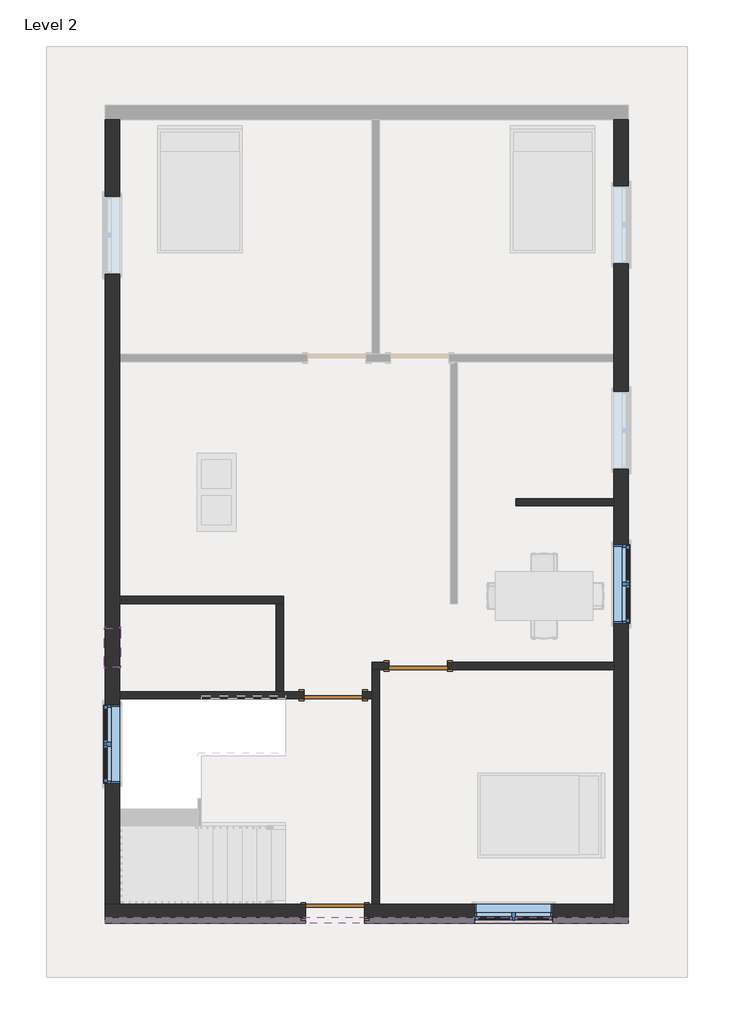
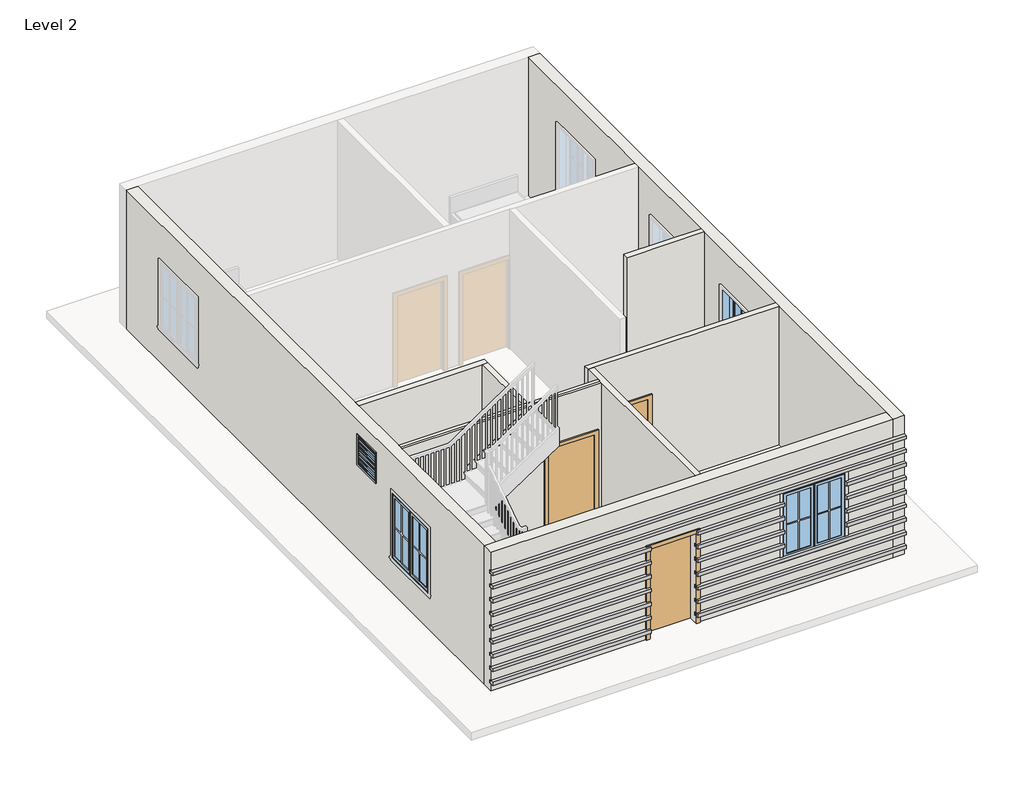
# One storey, part 1 of 3: 9 proxies, 9 walls, 4 windows, 3 doors.
"""IFC4 building model written with IfcOpenShell, lengths in millimetres."""

from ifc_helpers import new_model, si_unit, frame, origin, place, context, project, spatial, polyline, outline, extrude, faceted_brep, transform, mapped, element, save
from components import single_flush_door_3_17d80c48, single_flush_door_3_5e62189b, single_flush_door_3_89fc3733, window_casement_double_window_4_576b2d2c, window_f2d8fef0

model = new_model("IFC4")

# Units and contexts
model_context = context("Model", 3, world=origin())
ifc_project = project(units=[si_unit("LENGTHUNIT", "METRE", prefix="MILLI")], contexts=[model_context])

# Site, building, storey
site = spatial("IfcSite", under=ifc_project)
building = spatial("IfcBuilding", under=site)
storey = spatial("IfcBuildingStorey", under=building, Name="Level 2", Elevation=3048.0)

# Proxies
placement = place(None, origin())
element("IfcBuildingElementProxy", 1, Name="Reveal", ObjectType="Reveal", at=placement, inside=storey, context=model_context, shape_type="SweptSolid", body=[
    extrude(outline(polyline([(2831.4882597, -6585.4426559), (2831.4882597, -6677.5176559), (-1289.6617403, -6677.5176559), (-1289.6617403, -6585.4426559), (2831.4882597, -6585.4426559)])), frame((0.0, 0.0, 3352.8), z_axis=(0.0, 0.0, 1.0), x_axis=(1.0, 0.0, 0.0)), (0.0, 0.0, 1.0), 67.7333333),
    extrude(outline(polyline([(-2204.0617403, -6585.4426559), (-2204.0617403, -6677.5176559), (-5334.6117403, -6677.5176559), (-5334.6117403, -6585.4426559), (-2204.0617403, -6585.4426559)])), frame((0.0, 0.0, 3352.8), z_axis=(0.0, 0.0, 1.0), x_axis=(1.0, 0.0, 0.0)), (0.0, 0.0, 1.0), 67.7333333),
])
element("IfcBuildingElementProxy", 2, Name="Reveal", ObjectType="Reveal", at=placement, inside=storey, context=model_context, shape_type="SweptSolid", body=[
    extrude(outline(polyline([(2831.4882597, -6585.4426559), (2831.4882597, -6677.5176559), (-1289.6617403, -6677.5176559), (-1289.6617403, -6585.4426559), (2831.4882597, -6585.4426559)])), frame((0.0, 0.0, 3639.2994231), z_axis=(0.0, 0.0, 1.0), x_axis=(1.0, 0.0, 0.0)), (0.0, 0.0, 1.0), 67.7333333),
    extrude(outline(polyline([(-2204.0617403, -6585.4426559), (-2204.0617403, -6677.5176559), (-5334.6117403, -6677.5176559), (-5334.6117403, -6585.4426559), (-2204.0617403, -6585.4426559)])), frame((0.0, 0.0, 3639.2994231), z_axis=(0.0, 0.0, 1.0), x_axis=(1.0, 0.0, 0.0)), (0.0, 0.0, 1.0), 67.7333333),
])
element("IfcBuildingElementProxy", 3, Name="Reveal", ObjectType="Reveal", at=placement, inside=storey, context=model_context, shape_type="SweptSolid", body=[
    extrude(outline(polyline([(2831.4882597, -6585.4426559), (2831.4882597, -6677.5176559), (-1289.6617403, -6677.5176559), (-1289.6617403, -6585.4426559), (2831.4882597, -6585.4426559)])), frame((0.0, 0.0, 3925.7988461), z_axis=(0.0, 0.0, 1.0), x_axis=(1.0, 0.0, 0.0)), (0.0, 0.0, 1.0), 67.7333333),
    extrude(outline(polyline([(-2204.0617403, -6585.4426559), (-2204.0617403, -6677.5176559), (-5334.6117403, -6677.5176559), (-5334.6117403, -6585.4426559), (-2204.0617403, -6585.4426559)])), frame((0.0, 0.0, 3925.7988461), z_axis=(0.0, 0.0, 1.0), x_axis=(1.0, 0.0, 0.0)), (0.0, 0.0, 1.0), 67.7333333),
])
element("IfcBuildingElementProxy", 4, Name="Reveal", ObjectType="Reveal", at=placement, inside=storey, context=model_context, shape_type="SweptSolid", body=[
    extrude(outline(polyline([(2831.4882597, -6585.4426559), (2831.4882597, -6677.5176559), (1650.3882597, -6677.5176559), (1650.3882597, -6585.4426559), (2831.4882597, -6585.4426559)])), frame((0.0, 0.0, 4212.2982692), z_axis=(0.0, 0.0, 1.0), x_axis=(1.0, 0.0, 0.0)), (0.0, 0.0, 1.0), 67.7333333),
    extrude(outline(polyline([(431.1882597, -6585.4426559), (431.1882597, -6677.5176559), (-1289.6617403, -6677.5176559), (-1289.6617403, -6585.4426559), (431.1882597, -6585.4426559)])), frame((0.0, 0.0, 4212.2982692), z_axis=(0.0, 0.0, 1.0), x_axis=(1.0, 0.0, 0.0)), (0.0, 0.0, 1.0), 67.7333333),
    extrude(outline(polyline([(-2204.0617403, -6585.4426559), (-2204.0617403, -6677.5176559), (-5334.6117403, -6677.5176559), (-5334.6117403, -6585.4426559), (-2204.0617403, -6585.4426559)])), frame((0.0, 0.0, 4212.2982692), z_axis=(0.0, 0.0, 1.0), x_axis=(1.0, 0.0, 0.0)), (0.0, 0.0, 1.0), 67.7333333),
])
element("IfcBuildingElementProxy", 5, Name="Reveal", ObjectType="Reveal", at=placement, inside=storey, context=model_context, shape_type="SweptSolid", body=[
    extrude(outline(polyline([(2831.4882597, -6585.4426559), (2831.4882597, -6677.5176559), (1650.3882597, -6677.5176559), (1650.3882597, -6585.4426559), (2831.4882597, -6585.4426559)])), frame((0.0, 0.0, 4498.7976923), z_axis=(0.0, 0.0, 1.0), x_axis=(1.0, 0.0, 0.0)), (0.0, 0.0, 1.0), 67.7333333),
    extrude(outline(polyline([(431.1882597, -6585.4426559), (431.1882597, -6677.5176559), (-1289.6617403, -6677.5176559), (-1289.6617403, -6585.4426559), (431.1882597, -6585.4426559)])), frame((0.0, 0.0, 4498.7976923), z_axis=(0.0, 0.0, 1.0), x_axis=(1.0, 0.0, 0.0)), (0.0, 0.0, 1.0), 67.7333333),
    extrude(outline(polyline([(-2204.0617403, -6585.4426559), (-2204.0617403, -6677.5176559), (-5334.6117403, -6677.5176559), (-5334.6117403, -6585.4426559), (-2204.0617403, -6585.4426559)])), frame((0.0, 0.0, 4498.7976923), z_axis=(0.0, 0.0, 1.0), x_axis=(1.0, 0.0, 0.0)), (0.0, 0.0, 1.0), 67.7333333),
])
element("IfcBuildingElementProxy", 6, Name="Reveal", ObjectType="Reveal", at=placement, inside=storey, context=model_context, shape_type="SweptSolid", body=[
    extrude(outline(polyline([(2831.4882597, -6585.4426559), (2831.4882597, -6677.5176559), (1650.3882597, -6677.5176559), (1650.3882597, -6585.4426559), (2831.4882597, -6585.4426559)])), frame((0.0, 0.0, 4785.2971154), z_axis=(0.0, 0.0, 1.0), x_axis=(1.0, 0.0, 0.0)), (0.0, 0.0, 1.0), 67.7333333),
    extrude(outline(polyline([(431.1882597, -6585.4426559), (431.1882597, -6677.5176559), (-1289.6617403, -6677.5176559), (-1289.6617403, -6585.4426559), (431.1882597, -6585.4426559)])), frame((0.0, 0.0, 4785.2971154), z_axis=(0.0, 0.0, 1.0), x_axis=(1.0, 0.0, 0.0)), (0.0, 0.0, 1.0), 67.7333333),
    extrude(outline(polyline([(-2204.0617403, -6585.4426559), (-2204.0617403, -6677.5176559), (-5334.6117403, -6677.5176559), (-5334.6117403, -6585.4426559), (-2204.0617403, -6585.4426559)])), frame((0.0, 0.0, 4785.2971154), z_axis=(0.0, 0.0, 1.0), x_axis=(1.0, 0.0, 0.0)), (0.0, 0.0, 1.0), 67.7333333),
])
element("IfcBuildingElementProxy", 7, Name="Reveal", ObjectType="Reveal", at=placement, inside=storey, context=model_context, shape_type="SweptSolid", body=[
    extrude(outline(polyline([(2831.4882597, -6585.4426559), (2831.4882597, -6677.5176559), (1650.3882597, -6677.5176559), (1650.3882597, -6585.4426559), (2831.4882597, -6585.4426559)])), frame((0.0, 0.0, 5071.7965384), z_axis=(0.0, 0.0, 1.0), x_axis=(1.0, 0.0, 0.0)), (0.0, 0.0, 1.0), 67.7333333),
    extrude(outline(polyline([(431.1882597, -6585.4426559), (431.1882597, -6677.5176559), (-1289.6617403, -6677.5176559), (-1289.6617403, -6585.4426559), (431.1882597, -6585.4426559)])), frame((0.0, 0.0, 5071.7965384), z_axis=(0.0, 0.0, 1.0), x_axis=(1.0, 0.0, 0.0)), (0.0, 0.0, 1.0), 67.7333333),
    extrude(outline(polyline([(-2204.0617403, -6585.4426559), (-2204.0617403, -6677.5176559), (-5334.6117403, -6677.5176559), (-5334.6117403, -6585.4426559), (-2204.0617403, -6585.4426559)])), frame((0.0, 0.0, 5071.7965384), z_axis=(0.0, 0.0, 1.0), x_axis=(1.0, 0.0, 0.0)), (0.0, 0.0, 1.0), 67.7333333),
])
element("IfcBuildingElementProxy", 8, Name="Reveal", ObjectType="Reveal", at=placement, inside=storey, context=model_context, shape_type="SweptSolid", body=[
    extrude(outline(polyline([(2831.4882597, -6585.4426559), (2831.4882597, -6677.5176559), (-5334.6117403, -6677.5176559), (-5334.6117403, -6585.4426559), (2831.4882597, -6585.4426559)])), frame((0.0, 0.0, 5358.2959615), z_axis=(0.0, 0.0, 1.0), x_axis=(1.0, 0.0, 0.0)), (0.0, 0.0, 1.0), 67.7333333),
])
element("IfcBuildingElementProxy", 9, Name="Reveal", ObjectType="Reveal", at=placement, inside=storey, context=model_context, shape_type="SweptSolid", body=[
    extrude(outline(polyline([(2831.4882597, -6585.4426559), (2831.4882597, -6677.5176559), (-5334.6117403, -6677.5176559), (-5334.6117403, -6585.4426559), (2831.4882597, -6585.4426559)])), frame((0.0, 0.0, 5644.7953846), z_axis=(0.0, 0.0, 1.0), x_axis=(1.0, 0.0, 0.0)), (0.0, 0.0, 1.0), 67.7333333),
])

# Doors
single_flush_door_3_shape = single_flush_door_3_17d80c48(model_context)
element("IfcDoor", 10, ObjectType="Single-Flush : DOOR 3'", at=placement, inside=storey, context=model_context, shape_type="MappedRepresentation", body=[
    mapped(single_flush_door_3_shape, transform((-451.4617403, -2667.4926559, 3048.0), x_axis=(-1.0, 0.0, 0.0), y_axis=(0.0, -1.0, 0.0), z_axis=(0.0, 0.0, 1.0))),
])
single_flush_door_3_2_shape = single_flush_door_3_5e62189b(model_context)
element("IfcDoor", 11, ObjectType="Single-Flush : DOOR 3'", at=placement, inside=storey, context=model_context, shape_type="MappedRepresentation", body=[
    mapped(single_flush_door_3_2_shape, transform((-1772.2617403, -3124.6926559, 3048.0), x_axis=(1.0, 0.0, 0.0), y_axis=(0.0, 1.0, 0.0), z_axis=(0.0, 0.0, 1.0))),
])
single_flush_door_3_3_shape = single_flush_door_3_89fc3733(model_context)
element("IfcDoor", 12, ObjectType="Single-Flush : DOOR 3'", at=placement, inside=storey, context=model_context, shape_type="MappedRepresentation", body=[
    mapped(single_flush_door_3_3_shape, transform((-1746.8617403, -6496.5426559, 3048.0), x_axis=(1.0, 0.0, 0.0), y_axis=(0.0, 1.0, 0.0), z_axis=(0.0, 0.0, 1.0))),
])

# Walls
element("IfcWall", 13, ObjectType="ALL 4.5\"", at=placement, inside=storey, context=model_context, shape_type="SweptSolid", body=[
    extrude(outline(polyline([(1078.8882597, -57.6426559), (2602.8882597, -57.6426559), (2602.8882597, -171.9426559), (1078.8882597, -171.9426559), (1078.8882597, -57.6426559)])), frame((0.0, 0.0, 3048.0), z_axis=(0.0, 0.0, 1.0), x_axis=(1.0, 0.0, 0.0)), (0.0, 0.0, 1.0), 3048.0),
])
element("IfcWall", 14, ObjectType="ALL 4.5\"", at=placement, inside=storey, context=model_context, shape_type="Brep", body=[
    faceted_brep([(-908.6617403, -2610.3426559, 5080.0), (-908.6617403, -2610.3426559, 3048.0), (-1169.0117403, -2610.3426559, 3048.0), (-1169.0117403, -2610.3426559, 6096.0), (2602.8882597, -2610.3426559, 6096.0), (2602.8882597, -2610.3426559, 3048.0), (5.7382597, -2610.3426559, 3048.0), (5.7382597, -2610.3426559, 5080.0), (-1169.0117403, -2724.6426559, 3048.0), (-1054.7117403, -2724.6426559, 3048.0), (-908.6617403, -2724.6426559, 3048.0), (-908.6617403, -2724.6426559, 5080.0), (5.7382597, -2724.6426559, 5080.0), (5.7382597, -2724.6426559, 3048.0), (2602.8882597, -2724.6426559, 3048.0), (2602.8882597, -2724.6426559, 6096.0), (-1054.7117403, -2724.6426559, 6096.0), (-1169.0117403, -2724.6426559, 6096.0)], [[[0, 1, 2, 3, 4, 5, 6, 7]], [[8, 9, 10, 11, 12, 13, 14, 15, 16, 17]], [[6, 5, 14, 13]], [[2, 1, 10, 9, 8]], [[5, 4, 15, 14]], [[3, 2, 8, 17]], [[11, 10, 1, 0]], [[12, 11, 0, 7]], [[13, 12, 7, 6]], [[4, 3, 17, 16, 15]]]),
])
element("IfcWall", 15, ObjectType="ALL 4.5\"", at=placement, inside=storey, context=model_context, shape_type="Brep", body=[
    faceted_brep([(-1169.0117403, -2724.6426559, 3048.0), (-1169.0117403, -3067.5426559, 3048.0), (-1169.0117403, -3181.8426559, 3048.0), (-1169.0117403, -6382.2426559, 3048.0), (-1169.0117403, -6382.2426559, 6096.0), (-1169.0117403, -3181.8426559, 6096.0), (-1169.0117403, -3067.5426559, 6096.0), (-1169.0117403, -2724.6426559, 6096.0), (-1054.7117403, -2724.6426559, 3048.0), (-1054.7117403, -2724.6426559, 6096.0), (-1054.7117403, -6382.2426559, 6096.0), (-1054.7117403, -6382.2426559, 3048.0)], [[[0, 1, 2, 3, 4, 5, 6, 7]], [[8, 9, 10, 11]], [[3, 2, 1, 0, 8, 11]], [[0, 7, 9, 8]], [[4, 3, 11, 10]], [[7, 6, 5, 4, 10, 9]]]),
])
element("IfcWall", 16, ObjectType="ALL 4.5\"", at=placement, inside=storey, context=model_context, shape_type="Brep", body=[
    faceted_brep([(-1169.0117403, -3067.5426559, 3048.0), (-1315.0617403, -3067.5426559, 3048.0), (-1315.0617403, -3067.5426559, 5080.0), (-2229.4617403, -3067.5426559, 5080.0), (-2229.4617403, -3067.5426559, 3048.0), (-2553.3117403, -3067.5426559, 3048.0), (-2667.6117403, -3067.5426559, 3048.0), (-5106.0117403, -3067.5426559, 3048.0), (-5106.0117403, -3067.5426559, 6096.0), (-2667.6117403, -3067.5426559, 6096.0), (-2553.3117403, -3067.5426559, 6096.0), (-1169.0117403, -3067.5426559, 6096.0), (-1315.0617403, -3181.8426559, 5080.0), (-1315.0617403, -3181.8426559, 3048.0), (-1169.0117403, -3181.8426559, 3048.0), (-1169.0117403, -3181.8426559, 6096.0), (-5106.0117403, -3181.8426559, 6096.0), (-5106.0117403, -3181.8426559, 3048.0), (-2229.4617403, -3181.8426559, 3048.0), (-2229.4617403, -3181.8426559, 5080.0), (-5106.0117403, -3131.0426559, 6096.0), (-1169.0117403, -3131.0426559, 6096.0), (-2515.2117403, -3131.0426559, 6096.0)], [[[0, 1, 2, 3, 4, 5, 6, 7, 8, 9, 10, 11]], [[12, 13, 14, 15, 16, 17, 18, 19]], [[18, 17, 7, 6, 5, 4]], [[14, 13, 1, 0]], [[8, 7, 17, 16, 20]], [[0, 11, 21, 15, 14]], [[2, 1, 13, 12]], [[3, 2, 12, 19]], [[4, 3, 19, 18]], [[11, 10, 9, 8, 20, 22, 21]], [[20, 16, 15, 21, 22]]]),
])
element("IfcWall", 17, ObjectType="ALL 4.5\"", at=placement, inside=storey, context=model_context, shape_type="Brep", body=[
    faceted_brep([(-5106.0117403, -1695.9426559, 3048.0), (-2667.6117403, -1695.9426559, 3048.0), (-2553.3117403, -1695.9426559, 3048.0), (-2553.3117403, -1695.9426559, 6096.0), (-2667.6117403, -1695.9426559, 6096.0), (-5106.0117403, -1695.9426559, 6096.0), (-5106.0117403, -1581.6426559, 3048.0), (-5106.0117403, -1581.6426559, 6096.0), (-2553.3117403, -1581.6426559, 6096.0), (-2553.3117403, -1581.6426559, 3048.0)], [[[0, 1, 2, 3, 4, 5]], [[6, 7, 8, 9]], [[2, 1, 0, 6, 9]], [[0, 5, 7, 6]], [[3, 2, 9, 8]], [[5, 4, 3, 8, 7]]]),
])
element("IfcWall", 18, ObjectType="ALL 4.5\"", at=placement, inside=storey, context=model_context, shape_type="SweptSolid", body=[
    extrude(outline(polyline([(-2667.6117403, -3067.5426559), (-2667.6117403, -1695.9426559), (-2553.3117403, -1695.9426559), (-2553.3117403, -3067.5426559), (-2667.6117403, -3067.5426559)])), frame((0.0, 0.0, 3048.0), z_axis=(0.0, 0.0, 1.0), x_axis=(1.0, 0.0, 0.0)), (0.0, 0.0, 1.0), 3048.0),
])
element("IfcWall", 19, ObjectType="WALL 9\"", at=placement, inside=storey, context=model_context, shape_type="Brep", body=[
    faceted_brep([(2602.8882597, 5847.8573441, 3048.0), (2602.8882597, 2190.2573441, 3048.0), (2602.8882597, 2075.9573441, 3048.0), (2602.8882597, -57.6426559, 3048.0), (2602.8882597, -171.9426559, 3048.0), (2602.8882597, -2610.3426559, 3048.0), (2602.8882597, -2724.6426559, 3048.0), (2602.8882597, -6382.2426559, 3048.0), (2602.8882597, -6610.8426559, 3048.0), (2602.8882597, -6610.8426559, 3352.8), (2602.8882597, -6585.4426559, 3352.8), (2602.8882597, -6585.4426559, 3420.5333333), (2602.8882597, -6610.8426559, 3420.5333333), (2602.8882597, -6610.8426559, 3639.2994231), (2602.8882597, -6585.4426559, 3639.2994231), (2602.8882597, -6585.4426559, 3707.0327564), (2602.8882597, -6610.8426559, 3707.0327564), (2602.8882597, -6610.8426559, 3925.7988461), (2602.8882597, -6585.4426559, 3925.7988461), (2602.8882597, -6585.4426559, 3993.5321795), (2602.8882597, -6610.8426559, 3993.5321795), (2602.8882597, -6610.8426559, 4212.2982692), (2602.8882597, -6585.4426559, 4212.2982692), (2602.8882597, -6585.4426559, 4280.0316025), (2602.8882597, -6610.8426559, 4280.0316025), (2602.8882597, -6610.8426559, 4498.7976923), (2602.8882597, -6585.4426559, 4498.7976923), (2602.8882597, -6585.4426559, 4566.5310256), (2602.8882597, -6610.8426559, 4566.5310256), (2602.8882597, -6610.8426559, 4785.2971154), (2602.8882597, -6585.4426559, 4785.2971154), (2602.8882597, -6585.4426559, 4853.0304487), (2602.8882597, -6610.8426559, 4853.0304487), (2602.8882597, -6610.8426559, 5071.7965384), (2602.8882597, -6585.4426559, 5071.7965384), (2602.8882597, -6585.4426559, 5139.5298718), (2602.8882597, -6610.8426559, 5139.5298718), (2602.8882597, -6610.8426559, 5358.2959615), (2602.8882597, -6585.4426559, 5358.2959615), (2602.8882597, -6585.4426559, 5426.0292948), (2602.8882597, -6610.8426559, 5426.0292948), (2602.8882597, -6610.8426559, 5644.7953846), (2602.8882597, -6585.4426559, 5644.7953846), (2602.8882597, -6585.4426559, 5712.5287179), (2602.8882597, -6610.8426559, 5712.5287179), (2602.8882597, -6610.8426559, 6096.0), (2602.8882597, -6382.2426559, 6096.0), (2602.8882597, -2724.6426559, 6096.0), (2602.8882597, -2610.3426559, 6096.0), (2602.8882597, -171.9426559, 6096.0), (2602.8882597, -57.6426559, 6096.0), (2602.8882597, 2075.9573441, 6096.0), (2602.8882597, 2190.2573441, 6096.0), (2602.8882597, 5847.8573441, 6096.0), (2602.8882597, 3599.9573441, 5308.6), (2602.8882597, 3599.9573441, 3962.4), (2602.8882597, 4819.1573441, 3962.4), (2602.8882597, 4819.1573441, 5308.6), (2602.8882597, 399.5573441, 5308.6), (2602.8882597, 399.5573441, 3962.4), (2602.8882597, 1618.7573441, 3962.4), (2602.8882597, 1618.7573441, 5308.6), (2602.8882597, -2000.7426559, 5308.6), (2602.8882597, -2000.7426559, 3962.4), (2602.8882597, -781.5426559, 3962.4), (2602.8882597, -781.5426559, 5308.6), (2831.4882597, -6610.8426559, 3048.0), (2831.4882597, 5847.8573441, 3048.0), (2831.4882597, 5847.8573441, 6096.0), (2831.4882597, -6610.8426559, 6096.0), (2831.4882597, -6610.8426559, 5712.5287179), (2831.4882597, -6585.4426559, 5712.5287179), (2831.4882597, -6585.4426559, 5644.7953846), (2831.4882597, -6610.8426559, 5644.7953846), (2831.4882597, -6610.8426559, 5426.0292948), (2831.4882597, -6585.4426559, 5426.0292948), (2831.4882597, -6585.4426559, 5358.2959615), (2831.4882597, -6610.8426559, 5358.2959615), (2831.4882597, -6610.8426559, 5139.5298718), (2831.4882597, -6585.4426559, 5139.5298718), (2831.4882597, -6585.4426559, 5071.7965384), (2831.4882597, -6610.8426559, 5071.7965384), (2831.4882597, -6610.8426559, 4853.0304487), (2831.4882597, -6585.4426559, 4853.0304487), (2831.4882597, -6585.4426559, 4785.2971154), (2831.4882597, -6610.8426559, 4785.2971154), (2831.4882597, -6610.8426559, 4566.5310256), (2831.4882597, -6585.4426559, 4566.5310256), (2831.4882597, -6585.4426559, 4498.7976923), (2831.4882597, -6610.8426559, 4498.7976923), (2831.4882597, -6610.8426559, 4280.0316025), (2831.4882597, -6585.4426559, 4280.0316025), (2831.4882597, -6585.4426559, 4212.2982692), (2831.4882597, -6610.8426559, 4212.2982692), (2831.4882597, -6610.8426559, 3993.5321795), (2831.4882597, -6585.4426559, 3993.5321795), (2831.4882597, -6585.4426559, 3925.7988461), (2831.4882597, -6610.8426559, 3925.7988461), (2831.4882597, -6610.8426559, 3707.0327564), (2831.4882597, -6585.4426559, 3707.0327564), (2831.4882597, -6585.4426559, 3639.2994231), (2831.4882597, -6610.8426559, 3639.2994231), (2831.4882597, -6610.8426559, 3420.5333333), (2831.4882597, -6585.4426559, 3420.5333333), (2831.4882597, -6585.4426559, 3352.8), (2831.4882597, -6610.8426559, 3352.8), (2831.4882597, 3599.9573441, 3962.4), (2831.4882597, 3599.9573441, 5308.6), (2831.4882597, 4819.1573441, 5308.6), (2831.4882597, 4819.1573441, 3962.4), (2831.4882597, 399.5573441, 3962.4), (2831.4882597, 399.5573441, 5308.6), (2831.4882597, 1618.7573441, 5308.6), (2831.4882597, 1618.7573441, 3962.4), (2831.4882597, -2000.7426559, 3962.4), (2831.4882597, -2000.7426559, 5308.6), (2831.4882597, -781.5426559, 5308.6), (2831.4882597, -781.5426559, 3962.4)], [[[0, 1, 2, 3, 4, 5, 6, 7, 8, 9, 10, 11, 12, 13, 14, 15, 16, 17, 18, 19, 20, 21, 22, 23, 24, 25, 26, 27, 28, 29, 30, 31, 32, 33, 34, 35, 36, 37, 38, 39, 40, 41, 42, 43, 44, 45, 46, 47, 48, 49, 50, 51, 52, 53], [54, 55, 56, 57], [58, 59, 60, 61], [62, 63, 64, 65]], [[66, 67, 68, 69, 70, 71, 72, 73, 74, 75, 76, 77, 78, 79, 80, 81, 82, 83, 84, 85, 86, 87, 88, 89, 90, 91, 92, 93, 94, 95, 96, 97, 98, 99, 100, 101, 102, 103, 104, 105], [106, 107, 108, 109], [110, 111, 112, 113], [114, 115, 116, 117]], [[8, 7, 6, 5, 4, 3, 2, 1, 0, 67, 66]], [[0, 53, 68, 67]], [[8, 66, 105, 9]], [[69, 45, 44, 70]], [[12, 102, 101, 13]], [[16, 98, 97, 17]], [[20, 94, 93, 21]], [[24, 90, 89, 25]], [[28, 86, 85, 29]], [[32, 82, 81, 33]], [[36, 78, 77, 37]], [[40, 74, 73, 41]], [[55, 54, 107, 106]], [[56, 55, 106, 109]], [[57, 56, 109, 108]], [[54, 57, 108, 107]], [[59, 58, 111, 110]], [[60, 59, 110, 113]], [[61, 60, 113, 112]], [[58, 61, 112, 111]], [[63, 62, 115, 114]], [[64, 63, 114, 117]], [[65, 64, 117, 116]], [[62, 65, 116, 115]], [[53, 52, 51, 50, 49, 48, 47, 46, 45, 69, 68]], [[11, 103, 102, 12]], [[104, 10, 9, 105]], [[103, 11, 10, 104]], [[15, 99, 98, 16]], [[100, 14, 13, 101]], [[99, 15, 14, 100]], [[19, 95, 94, 20]], [[96, 18, 17, 97]], [[95, 19, 18, 96]], [[23, 91, 90, 24]], [[92, 22, 21, 93]], [[91, 23, 22, 92]], [[27, 87, 86, 28]], [[88, 26, 25, 89]], [[87, 27, 26, 88]], [[31, 83, 82, 32]], [[84, 30, 29, 85]], [[83, 31, 30, 84]], [[35, 79, 78, 36]], [[80, 34, 33, 81]], [[79, 35, 34, 80]], [[39, 75, 74, 40]], [[76, 38, 37, 77]], [[75, 39, 38, 76]], [[43, 71, 70, 44]], [[72, 42, 41, 73]], [[71, 43, 42, 72]]]),
])
element("IfcWall", 20, ObjectType="WALL 9\"", at=placement, inside=storey, context=model_context, shape_type="Brep", body=[
    faceted_brep([(-5334.6117403, -6382.2426559, 6096.0), (-5106.0117403, -6382.2426559, 6096.0), (-1169.0117403, -6382.2426559, 6096.0), (-1054.7117403, -6382.2426559, 6096.0), (2602.8882597, -6382.2426559, 6096.0), (2602.8882597, -6382.2426559, 3048.0), (-1054.7117403, -6382.2426559, 3048.0), (-1169.0117403, -6382.2426559, 3048.0), (-1289.6617403, -6382.2426559, 3048.0), (-1289.6617403, -6382.2426559, 5080.0), (-2204.0617403, -6382.2426559, 5080.0), (-2204.0617403, -6382.2426559, 3048.0), (-5106.0117403, -6382.2426559, 3048.0), (-5334.6117403, -6382.2426559, 3048.0), (431.1882597, -6382.2426559, 5308.6), (431.1882597, -6382.2426559, 3962.4), (1650.3882597, -6382.2426559, 3962.4), (1650.3882597, -6382.2426559, 5308.6), (2602.8882597, -6610.8426559, 6096.0), (-5334.6117403, -6610.8426559, 6096.0), (-5334.6117403, -6610.8426559, 5712.5287179), (2602.8882597, -6610.8426559, 5712.5287179), (431.1882597, -6610.8426559, 5308.6), (1650.3882597, -6610.8426559, 5308.6), (1650.3882597, -6610.8426559, 5139.5298718), (2602.8882597, -6610.8426559, 5139.5298718), (2602.8882597, -6610.8426559, 5358.2959615), (-5334.6117403, -6610.8426559, 5358.2959615), (-5334.6117403, -6610.8426559, 5139.5298718), (-2204.0617403, -6610.8426559, 5139.5298718), (-2204.0617403, -6610.8426559, 5080.0), (-1289.6617403, -6610.8426559, 5080.0), (-1289.6617403, -6610.8426559, 5139.5298718), (431.1882597, -6610.8426559, 5139.5298718), (-5334.6117403, -6610.8426559, 3048.0), (-2204.0617403, -6610.8426559, 3048.0), (-2204.0617403, -6610.8426559, 3352.8), (-5334.6117403, -6610.8426559, 3352.8), (-1289.6617403, -6610.8426559, 3048.0), (2602.8882597, -6610.8426559, 3048.0), (2602.8882597, -6610.8426559, 3352.8), (-1289.6617403, -6610.8426559, 3352.8), (-1289.6617403, -6610.8426559, 3420.5333333), (2602.8882597, -6610.8426559, 3420.5333333), (2602.8882597, -6610.8426559, 3639.2994231), (-1289.6617403, -6610.8426559, 3639.2994231), (-5334.6117403, -6610.8426559, 3420.5333333), (-2204.0617403, -6610.8426559, 3420.5333333), (-2204.0617403, -6610.8426559, 3639.2994231), (-5334.6117403, -6610.8426559, 3639.2994231), (-1289.6617403, -6610.8426559, 3707.0327564), (2602.8882597, -6610.8426559, 3707.0327564), (2602.8882597, -6610.8426559, 3925.7988461), (-1289.6617403, -6610.8426559, 3925.7988461), (-5334.6117403, -6610.8426559, 3707.0327564), (-2204.0617403, -6610.8426559, 3707.0327564), (-2204.0617403, -6610.8426559, 3925.7988461), (-5334.6117403, -6610.8426559, 3925.7988461), (-1289.6617403, -6610.8426559, 3993.5321795), (431.1882597, -6610.8426559, 3993.5321795), (431.1882597, -6610.8426559, 4212.2982692), (-1289.6617403, -6610.8426559, 4212.2982692), (1650.3882597, -6610.8426559, 3993.5321795), (2602.8882597, -6610.8426559, 3993.5321795), (2602.8882597, -6610.8426559, 4212.2982692), (1650.3882597, -6610.8426559, 4212.2982692), (-5334.6117403, -6610.8426559, 3993.5321795), (-2204.0617403, -6610.8426559, 3993.5321795), (-2204.0617403, -6610.8426559, 4212.2982692), (-5334.6117403, -6610.8426559, 4212.2982692), (1650.3882597, -6610.8426559, 4280.0316025), (2602.8882597, -6610.8426559, 4280.0316025), (2602.8882597, -6610.8426559, 4498.7976923), (1650.3882597, -6610.8426559, 4498.7976923), (-1289.6617403, -6610.8426559, 4280.0316025), (431.1882597, -6610.8426559, 4280.0316025), (431.1882597, -6610.8426559, 4498.7976923), (-1289.6617403, -6610.8426559, 4498.7976923), (-5334.6117403, -6610.8426559, 4280.0316025), (-2204.0617403, -6610.8426559, 4280.0316025), (-2204.0617403, -6610.8426559, 4498.7976923), (-5334.6117403, -6610.8426559, 4498.7976923), (1650.3882597, -6610.8426559, 4566.5310256), (2602.8882597, -6610.8426559, 4566.5310256), (2602.8882597, -6610.8426559, 4785.2971154), (1650.3882597, -6610.8426559, 4785.2971154), (-1289.6617403, -6610.8426559, 4566.5310256), (431.1882597, -6610.8426559, 4566.5310256), (431.1882597, -6610.8426559, 4785.2971154), (-1289.6617403, -6610.8426559, 4785.2971154), (-5334.6117403, -6610.8426559, 4566.5310256), (-2204.0617403, -6610.8426559, 4566.5310256), (-2204.0617403, -6610.8426559, 4785.2971154), (-5334.6117403, -6610.8426559, 4785.2971154), (1650.3882597, -6610.8426559, 4853.0304487), (2602.8882597, -6610.8426559, 4853.0304487), (2602.8882597, -6610.8426559, 5071.7965384), (1650.3882597, -6610.8426559, 5071.7965384), (-1289.6617403, -6610.8426559, 4853.0304487), (431.1882597, -6610.8426559, 4853.0304487), (431.1882597, -6610.8426559, 5071.7965384), (-1289.6617403, -6610.8426559, 5071.7965384), (-5334.6117403, -6610.8426559, 4853.0304487), (-2204.0617403, -6610.8426559, 4853.0304487), (-2204.0617403, -6610.8426559, 5071.7965384), (-5334.6117403, -6610.8426559, 5071.7965384), (-5334.6117403, -6610.8426559, 5426.0292948), (2602.8882597, -6610.8426559, 5426.0292948), (2602.8882597, -6610.8426559, 5644.7953846), (-5334.6117403, -6610.8426559, 5644.7953846), (2602.8882597, -6585.4426559, 5712.5287179), (2602.8882597, -6585.4426559, 5644.7953846), (2602.8882597, -6585.4426559, 5426.0292948), (2602.8882597, -6585.4426559, 5358.2959615), (2602.8882597, -6585.4426559, 5139.5298718), (2602.8882597, -6585.4426559, 5071.7965384), (2602.8882597, -6585.4426559, 4853.0304487), (2602.8882597, -6585.4426559, 4785.2971154), (2602.8882597, -6585.4426559, 4566.5310256), (2602.8882597, -6585.4426559, 4498.7976923), (2602.8882597, -6585.4426559, 4280.0316025), (2602.8882597, -6585.4426559, 4212.2982692), (2602.8882597, -6585.4426559, 3993.5321795), (2602.8882597, -6585.4426559, 3925.7988461), (2602.8882597, -6585.4426559, 3707.0327564), (2602.8882597, -6585.4426559, 3639.2994231), (2602.8882597, -6585.4426559, 3420.5333333), (2602.8882597, -6585.4426559, 3352.8), (-5334.6117403, -6585.4426559, 3352.8), (-5334.6117403, -6585.4426559, 3420.5333333), (-5334.6117403, -6585.4426559, 3639.2994231), (-5334.6117403, -6585.4426559, 3707.0327564), (-5334.6117403, -6585.4426559, 3925.7988461), (-5334.6117403, -6585.4426559, 3993.5321795), (-5334.6117403, -6585.4426559, 4212.2982692), (-5334.6117403, -6585.4426559, 4280.0316025), (-5334.6117403, -6585.4426559, 4498.7976923), (-5334.6117403, -6585.4426559, 4566.5310256), (-5334.6117403, -6585.4426559, 4785.2971154), (-5334.6117403, -6585.4426559, 4853.0304487), (-5334.6117403, -6585.4426559, 5071.7965384), (-5334.6117403, -6585.4426559, 5139.5298718), (-5334.6117403, -6585.4426559, 5358.2959615), (-5334.6117403, -6585.4426559, 5426.0292948), (-5334.6117403, -6585.4426559, 5644.7953846), (-5334.6117403, -6585.4426559, 5712.5287179), (431.1882597, -6585.4426559, 5139.5298718), (431.1882597, -6585.4426559, 5071.7965384), (431.1882597, -6585.4426559, 4853.0304487), (431.1882597, -6585.4426559, 4785.2971154), (431.1882597, -6585.4426559, 4566.5310256), (431.1882597, -6585.4426559, 4498.7976923), (431.1882597, -6585.4426559, 4280.0316025), (431.1882597, -6585.4426559, 4212.2982692), (431.1882597, -6585.4426559, 3993.5321795), (431.1882597, -6585.4426559, 3962.4), (1650.3882597, -6585.4426559, 3962.4), (1650.3882597, -6585.4426559, 3993.5321795), (1650.3882597, -6585.4426559, 4212.2982692), (1650.3882597, -6585.4426559, 4280.0316025), (1650.3882597, -6585.4426559, 4498.7976923), (1650.3882597, -6585.4426559, 4566.5310256), (1650.3882597, -6585.4426559, 4785.2971154), (1650.3882597, -6585.4426559, 4853.0304487), (1650.3882597, -6585.4426559, 5071.7965384), (1650.3882597, -6585.4426559, 5139.5298718), (-1289.6617403, -6585.4426559, 3352.8), (-1289.6617403, -6585.4426559, 3420.5333333), (-1289.6617403, -6585.4426559, 3639.2994231), (-1289.6617403, -6585.4426559, 3707.0327564), (-1289.6617403, -6585.4426559, 3925.7988461), (-1289.6617403, -6585.4426559, 3993.5321795), (-1289.6617403, -6585.4426559, 4212.2982692), (-1289.6617403, -6585.4426559, 4280.0316025), (-1289.6617403, -6585.4426559, 4498.7976923), (-1289.6617403, -6585.4426559, 4566.5310256), (-1289.6617403, -6585.4426559, 4785.2971154), (-1289.6617403, -6585.4426559, 4853.0304487), (-1289.6617403, -6585.4426559, 5071.7965384), (-1289.6617403, -6585.4426559, 5080.0), (-2204.0617403, -6585.4426559, 5080.0), (-2204.0617403, -6585.4426559, 5071.7965384), (-2204.0617403, -6585.4426559, 4853.0304487), (-2204.0617403, -6585.4426559, 4785.2971154), (-2204.0617403, -6585.4426559, 4566.5310256), (-2204.0617403, -6585.4426559, 4498.7976923), (-2204.0617403, -6585.4426559, 4280.0316025), (-2204.0617403, -6585.4426559, 4212.2982692), (-2204.0617403, -6585.4426559, 3993.5321795), (-2204.0617403, -6585.4426559, 3925.7988461), (-2204.0617403, -6585.4426559, 3707.0327564), (-2204.0617403, -6585.4426559, 3639.2994231), (-2204.0617403, -6585.4426559, 3420.5333333), (-2204.0617403, -6585.4426559, 3352.8), (-1289.6617403, -6585.4426559, 5139.5298718), (-2204.0617403, -6585.4426559, 5139.5298718)], [[[0, 1, 2, 3, 4, 5, 6, 7, 8, 9, 10, 11, 12, 13], [14, 15, 16, 17]], [[18, 19, 20, 21]], [[22, 23, 24, 25, 26, 27, 28, 29, 30, 31, 32, 33]], [[34, 35, 36, 37]], [[38, 39, 40, 41]], [[42, 43, 44, 45]], [[46, 47, 48, 49]], [[50, 51, 52, 53]], [[54, 55, 56, 57]], [[58, 59, 60, 61]], [[62, 63, 64, 65]], [[66, 67, 68, 69]], [[70, 71, 72, 73]], [[74, 75, 76, 77]], [[78, 79, 80, 81]], [[82, 83, 84, 85]], [[86, 87, 88, 89]], [[90, 91, 92, 93]], [[94, 95, 96, 97]], [[98, 99, 100, 101]], [[102, 103, 104, 105]], [[106, 107, 108, 109]], [[5, 39, 38, 8, 7, 6]], [[34, 13, 12, 11, 35]], [[4, 3, 2, 1, 0, 19, 18]], [[5, 4, 18, 21, 110, 111, 108, 107, 112, 113, 26, 25, 114, 115, 96, 95, 116, 117, 84, 83, 118, 119, 72, 71, 120, 121, 64, 63, 122, 123, 52, 51, 124, 125, 44, 43, 126, 127, 40, 39]], [[0, 13, 34, 37, 128, 129, 46, 49, 130, 131, 54, 57, 132, 133, 66, 69, 134, 135, 78, 81, 136, 137, 90, 93, 138, 139, 102, 105, 140, 141, 28, 27, 142, 143, 106, 109, 144, 145, 20, 19]], [[15, 14, 22, 33, 146, 147, 100, 99, 148, 149, 88, 87, 150, 151, 76, 75, 152, 153, 60, 59, 154, 155]], [[16, 15, 155, 156]], [[17, 16, 156, 157, 62, 65, 158, 159, 70, 73, 160, 161, 82, 85, 162, 163, 94, 97, 164, 165, 24, 23]], [[14, 17, 23, 22]], [[9, 8, 38, 41, 166, 167, 42, 45, 168, 169, 50, 53, 170, 171, 58, 61, 172, 173, 74, 77, 174, 175, 86, 89, 176, 177, 98, 101, 178, 179]], [[10, 9, 179, 31, 30, 180]], [[11, 10, 180, 181, 104, 103, 182, 183, 92, 91, 184, 185, 80, 79, 186, 187, 68, 67, 188, 189, 56, 55, 190, 191, 48, 47, 192, 193, 36, 35]], [[167, 126, 43, 42]], [[127, 166, 41, 40]], [[126, 167, 166, 127]], [[129, 192, 47, 46]], [[193, 128, 37, 36]], [[192, 129, 128, 193]], [[169, 124, 51, 50]], [[125, 168, 45, 44]], [[124, 169, 168, 125]], [[131, 190, 55, 54]], [[191, 130, 49, 48]], [[190, 131, 130, 191]], [[171, 154, 59, 58]], [[157, 122, 63, 62]], [[123, 170, 53, 52]], [[154, 171, 170, 123, 122, 157, 156, 155]], [[133, 188, 67, 66]], [[189, 132, 57, 56]], [[188, 133, 132, 189]], [[159, 120, 71, 70]], [[121, 158, 65, 64]], [[120, 159, 158, 121]], [[173, 152, 75, 74]], [[153, 172, 61, 60]], [[152, 173, 172, 153]], [[135, 186, 79, 78]], [[187, 134, 69, 68]], [[186, 135, 134, 187]], [[161, 118, 83, 82]], [[119, 160, 73, 72]], [[118, 161, 160, 119]], [[175, 150, 87, 86]], [[151, 174, 77, 76]], [[150, 175, 174, 151]], [[137, 184, 91, 90]], [[185, 136, 81, 80]], [[184, 137, 136, 185]], [[163, 116, 95, 94]], [[117, 162, 85, 84]], [[116, 163, 162, 117]], [[177, 148, 99, 98]], [[149, 176, 89, 88]], [[148, 177, 176, 149]], [[139, 182, 103, 102]], [[183, 138, 93, 92]], [[182, 139, 138, 183]], [[165, 114, 25, 24]], [[115, 164, 97, 96]], [[114, 165, 164, 115]], [[179, 194, 32, 31]], [[194, 146, 33, 32]], [[147, 178, 101, 100]], [[146, 194, 179, 178, 147]], [[195, 180, 30, 29]], [[141, 195, 29, 28]], [[181, 140, 105, 104]], [[195, 141, 140, 181, 180]], [[143, 112, 107, 106]], [[113, 142, 27, 26]], [[112, 143, 142, 113]], [[145, 110, 21, 20]], [[111, 144, 109, 108]], [[110, 145, 144, 111]]]),
])
element("IfcWall", 21, ObjectType="WALL 9\"", at=placement, inside=storey, context=model_context, shape_type="Brep", body=[
    faceted_brep([(-5106.0117403, -6382.2426559, 3048.0), (-5106.0117403, -3181.8426559, 3048.0), (-5106.0117403, -3067.5426559, 3048.0), (-5106.0117403, -1695.9426559, 3048.0), (-5106.0117403, -1581.6426559, 3048.0), (-5106.0117403, 2075.9573441, 3048.0), (-5106.0117403, 2190.2573441, 3048.0), (-5106.0117403, 5847.8573441, 3048.0), (-5106.0117403, 5847.8573441, 6096.0), (-5106.0117403, 2190.2573441, 6096.0), (-5106.0117403, 2075.9573441, 6096.0), (-5106.0117403, -1581.6426559, 6096.0), (-5106.0117403, -1695.9426559, 6096.0), (-5106.0117403, -3067.5426559, 6096.0), (-5106.0117403, -3181.8426559, 6096.0), (-5106.0117403, -6382.2426559, 6096.0), (-5106.0117403, -3277.0926559, 5308.6), (-5106.0117403, -3277.0926559, 3962.4), (-5106.0117403, -4496.2926559, 3962.4), (-5106.0117403, -4496.2926559, 5308.6), (-5106.0117403, 4657.2323441, 5308.6), (-5106.0117403, 4657.2323441, 3962.4), (-5106.0117403, 3438.0323441, 3962.4), (-5106.0117403, 3438.0323441, 5308.6), (-5106.0117403, -2686.5426559, 5791.2), (-5106.0117403, -2076.9426559, 5791.2), (-5106.0117403, -2076.9426559, 5181.6), (-5106.0117403, -2686.5426559, 5181.6), (-5334.6117403, -6382.2426559, 3048.0), (-5334.6117403, -6382.2426559, 6096.0), (-5334.6117403, 5847.8573441, 6096.0), (-5334.6117403, 5847.8573441, 3048.0), (-5334.6117403, -3277.0926559, 5308.6), (-5334.6117403, -4496.2926559, 5308.6), (-5334.6117403, -4496.2926559, 3962.4), (-5334.6117403, -3277.0926559, 3962.4), (-5334.6117403, 4657.2323441, 5308.6), (-5334.6117403, 3438.0323441, 5308.6), (-5334.6117403, 3438.0323441, 3962.4), (-5334.6117403, 4657.2323441, 3962.4), (-5334.6117403, -2686.5426559, 5791.2), (-5334.6117403, -2686.5426559, 5181.6), (-5334.6117403, -2076.9426559, 5181.6), (-5334.6117403, -2076.9426559, 5791.2)], [[[0, 1, 2, 3, 4, 5, 6, 7, 8, 9, 10, 11, 12, 13, 14, 15], [16, 17, 18, 19], [20, 21, 22, 23], [24, 25, 26, 27]], [[28, 29, 30, 31], [32, 33, 34, 35], [36, 37, 38, 39], [40, 41, 42, 43]], [[7, 6, 5, 4, 3, 2, 1, 0, 28, 31]], [[15, 14, 13, 12, 11, 10, 9, 8, 30, 29]], [[8, 7, 31, 30]], [[0, 15, 29, 28]], [[17, 16, 32, 35]], [[18, 17, 35, 34]], [[19, 18, 34, 33]], [[16, 19, 33, 32]], [[21, 20, 36, 39]], [[22, 21, 39, 38]], [[23, 22, 38, 37]], [[20, 23, 37, 36]], [[41, 40, 24, 27]], [[42, 41, 27, 26]], [[43, 42, 26, 25]], [[40, 43, 25, 24]]]),
])

# Windows
window_casement_double_window_4_shape = window_casement_double_window_4_576b2d2c(model_context)
element("IfcWindow", 22, ObjectType="Window-Casement-Double : WINDOW 4'", at=placement, inside=storey, context=model_context, shape_type="MappedRepresentation", body=[
    mapped(window_casement_double_window_4_shape, transform((-5220.3117403, -3886.6926559, 3048.0), x_axis=(0.0, 1.0, 0.0), y_axis=(-1.0, 0.0, 0.0), z_axis=(0.0, 0.0, 1.0))),
])
element("IfcWindow", 23, ObjectType="Window-Casement-Double : WINDOW 4'", at=placement, inside=storey, context=model_context, shape_type="MappedRepresentation", body=[
    mapped(window_casement_double_window_4_shape, transform((2717.1882597, -1391.1426559, 3048.0), x_axis=(0.0, -1.0, 0.0), y_axis=(1.0, 0.0, 0.0), z_axis=(0.0, 0.0, 1.0))),
])
element("IfcWindow", 24, ObjectType="Window-Casement-Double : WINDOW 4'", at=placement, inside=storey, context=model_context, shape_type="MappedRepresentation", body=[
    mapped(window_casement_double_window_4_shape, transform((1040.7882597, -6496.5426559, 3048.0), x_axis=(-1.0, 0.0, 0.0), y_axis=(0.0, -1.0, 0.0), z_axis=(0.0, 0.0, 1.0))),
])
window_shape = window_f2d8fef0(model_context)
element("IfcWindow", 25, ObjectType="Window-Louvers : 24\" x 24\"", at=placement, inside=storey, context=model_context, shape_type="MappedRepresentation", body=[
    mapped(window_shape, transform((-5226.6617403, -2381.7426559, 4267.2), x_axis=(0.0, 1.0, 0.0), y_axis=(-1.0, 0.0, 0.0), z_axis=(0.0, 0.0, 1.0))),
])

save(model, "model.ifc")

# Revit data of these elements
# Type "Single-Flush : DOOR 3'"
#   Type Mark = "8"
#   Construction Type Id = "MDOOR"
#   Assembly Code = "C1020"
#   Analytic Construction = "Metal"
#   Thickness = 0' - 2"
#   Heat Transfer Coefficient (U) = 0.651978 BTU/(h·ft²·°F)
#   Height = 6' - 8"
#   Trim Projection Ext = 0' - 1"
#   Trim Projection Int = 0' - 1"
#   Trim Width = 0' - 3"
#   Width = 3' - 0"
#   Define Thermal Properties by = 1
#   Door Material = Door - Panel
#   Frame Material = Door - Frame
#   Visual Light Transmittance = 0
#   Solar Heat Gain Coefficient = 0
#   Function = (empty or 0)
#   Wall Closure = (empty or 0)
# Type "ALL 4.5\""
#   Assembly Code = "B2010"
#   Layers, outside or top first: 0' - 4 1/2" no material (function 1)
# Type "WALL 9\""
#   Assembly Code = "B2010"
#   Layers, outside or top first: 0' - 9" "Carpet (1)" (function 1)
# Type "Window-Casement-Double : WINDOW 4'"
#   Type Mark = "18"
#   Fire Rating = "0.5h"
#   Assembly Code = "B2020100"
#   Analytic Construction = "Double glazing - domestic"
#   Frame Extension [instance default] = 0' - 0 1/4"
#   Window Inset [instance default] = 0' - 0"
#   Wall Thickness [instance default] = 0' - 6"
#   Interior Wall Closure [instance default] = 0' - 2 1/4"
#   Half Width = 2' - 0"
#   Visual Light Transmittance = 0.81
#   Thermal Resistance (R) = 1.8146 (h·ft²·°F)/BTU
#   Solar Heat Gain Coefficient = 0.76
#   Rough Width = 4' - 0 1/2"
#   Rough Height = 4' - 5 1/2"
#   Height = 4' - 5"
#   Heat Transfer Coefficient (U) = 0.5511 BTU/(h·ft²·°F)
#   Exterior Wall Closure [instance default] = 0' - 1 1/4"
#   Extension Jamb [instance default] = 0' - 2 1/4"
#   Default Sill Height = 3' - 0"
#   Width = 4' - 0"
#   Muntin Visibility = yes
#   Interior Trim Visibility [instance default] = yes
#   Exterior Trim Visibility [instance default] = yes
#   Extension Jamb Visibility [instance default] = yes
#   Interior Trim Material = Wood - Stained
#   Muntin Pattern = Muntin Pattern_2x2 : Muntin Pattern_2x2
#   Interior Trim = Trim-Window-Interior-Flat : Picture Frame
#   Interior Frame Material = Wood - Stained
#   Glass Panel Material = Glass
#   Exterior Trim Material = Clad - White
#   Exterior Trim = Trim-Window-Exterior-Flat : with Sill
#   Exterior Frame Material = Clad - White
#   Wall Closure = (empty or 0)
# Type "Window-Louvers : 24\" x 24\""
#   Type Mark = "19"
#   Construction Type Id = "GSP4R"
#   Assembly Code = "B20"
#   Analytic Construction = "1/8 in Pilkington single glazing"
#   Visual Light Transmittance = 0.9
#   Thermal Resistance (R) = 1.53941 (h·ft²·°F)/BTU
#   Solar Heat Gain Coefficient = 0.78
#   Max Height = 1' - 11.74264"
#   Height = 2' - 0"
#   Heat Transfer Coefficient (U) = 0.6496 BTU/(h·ft²·°F)
#   Blade Width [instance default] = 1' - 10 1/2"
#   Blade Vertical Thickness = 0' - 0.35355"
#   Blade Thickness = 0' - 0 1/4"
#   Blade Spacing = 0' - 1 1/2"
#   Blade Height = 0' - 1.85355"
#   Blade Depth = 0' - 3"
#   Blade Angle = 45.00°
#   Default Sill Height = 3' - 0"
#   Trim Projection_Exterior = 0' - 0 1/2"
#   Trim Projection_Interior = 0' - 0 1/2"
#   Trim Width_Exterior = 0' - 1 1/2"
#   Trim Width_Interior = 0' - 1 1/2"
#   Width = 2' - 0"
#   Max Blade Count = 12
#   Define Thermal Properties by = 1
#   Blade Count = 12
#   Frame Material = Birch
#   Louver Material = Birch
#   Trim Exterior Material = Birch
#   Trim Interior Material = Birch
#   Wall Closure = (empty or 0)
# Elements 10, 11, 12 (IfcDoor, "Single-Flush : DOOR 3'")
#   Phase Created = New Construction
#   Materials on its faces: "Door - Frame", "Door - Panel"
# Elements 13, 17, 18 (IfcWall, "ALL 4.5\"")
#   Top Offset = 0' - 0"
#   Base Offset = 0' - 0"
#   Unconnected Height = 10' - 0"
#   wall height = 10' - 0"
#   Phase Created = New Construction
#   Base Constraint = Level 2
#   Materials on its faces: "Default Wall"
# Elements 14, 15, 16 (IfcWall, "ALL 4.5\"")
#   Top Offset = 0' - 0"
#   Base Offset = 0' - 0"
#   Unconnected Height = 10' - 0"
#   wall height = 10' - 0"
#   Phase Created = New Construction
#   Base Constraint = Level 2
#   Materials on its faces: "Default Wall", "Clad - White"
# Element 19 (IfcWall, "WALL 9\"")
#   Top Offset = 0' - 0"
#   Base Offset = 0' - 0"
#   Unconnected Height = 10' - 0"
#   wall height = 10' - 0"
#   Phase Created = New Construction
#   Base Constraint = Level 2
#   Materials on its faces: "Carpet (1)", "Wood - Stained"
# Elements 20, 21 (IfcWall, "WALL 9\"")
#   Top Offset = 0' - 0"
#   Base Offset = 0' - 0"
#   Unconnected Height = 10' - 0"
#   wall height = 10' - 0"
#   Phase Created = New Construction
#   Base Constraint = Level 2
#   Materials on its faces: "Carpet (1)", "Clad - White", "Wood - Stained"
# Element 22 (IfcWindow, "Window-Casement-Double : WINDOW 4'")
#   Mark = "8"
#   Window Inset = 0' - 0"
#   Interior Wall Closure = 0' - 2 1/4"
#   Frame Extension = 0' - 0 1/4"
#   Exterior Wall Closure = 0' - 1 1/4"
#   Interior Trim Visibility = yes
#   Exterior Trim Visibility = yes
#   Phase Created = New Construction
#   Materials on its faces: "Wood - Stained", "Glass", "Clad - White"
# Element 23 (IfcWindow, "Window-Casement-Double : WINDOW 4'")
#   Mark = "12"
#   Window Inset = 0' - 0"
#   Interior Wall Closure = 0' - 2 1/4"
#   Frame Extension = 0' - 0 1/4"
#   Exterior Wall Closure = 0' - 1 1/4"
#   Interior Trim Visibility = yes
#   Exterior Trim Visibility = yes
#   Phase Created = New Construction
#   Materials on its faces: "Wood - Stained", "Glass", "Clad - White"
# Element 24 (IfcWindow, "Window-Casement-Double : WINDOW 4'")
#   Mark = "13"
#   Window Inset = 0' - 0"
#   Interior Wall Closure = 0' - 2 1/4"
#   Frame Extension = 0' - 0 1/4"
#   Exterior Wall Closure = 0' - 1 1/4"
#   Interior Trim Visibility = yes
#   Exterior Trim Visibility = yes
#   Phase Created = New Construction
#   Materials on its faces: "Wood - Stained", "Glass", "Clad - White"
# Element 25 (IfcWindow, "Window-Louvers : 24\" x 24\"")
#   Mark = "14"
#   Blade Width = 1' - 10 1/2"
#   Phase Created = New Construction
#   Materials on its faces: "Birch"
# Materials
#   "Door - Panel": class "Wood", colour RGB 210 159 95, transparency 0, Cost = 0
#   "Door - Frame": colour RGB 118 70 51, transparency 0, Cost = 0
#   "Carpet (1)": class "Carpet", colour RGB 124 80 67, transparency 0, Description = "Interior finish", Cost = 0
#   "Wood - Stained": class "Wood", colour RGB 224 178 126, transparency 0, Cost = 0
#   "Glass": class "Glass", colour RGB 0 128 192, transparency 0.75, Description = "Soda Lime Glass", Cost = 0
#   "Clad - White": class "Wood", colour RGB 242 242 238, transparency 0, Cost = 0
#   "Birch": class "Wood", colour RGB 224 178 126, transparency 0, Description = "Betula Alleghaniensis", Cost = 0
#   "Default Wall": colour RGB 128 128 128, transparency 0, Cost = 0
